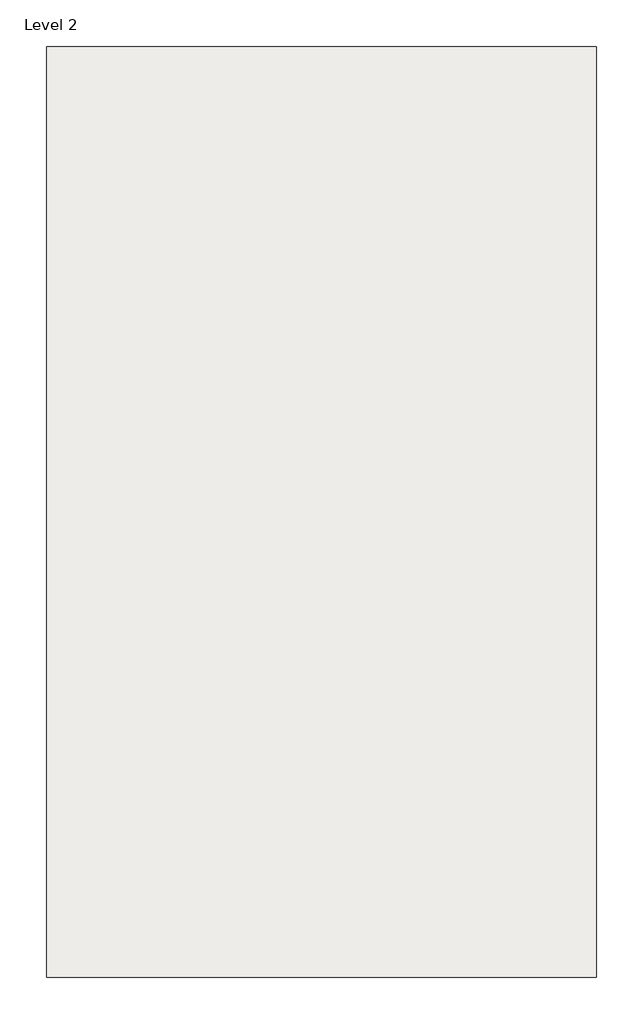
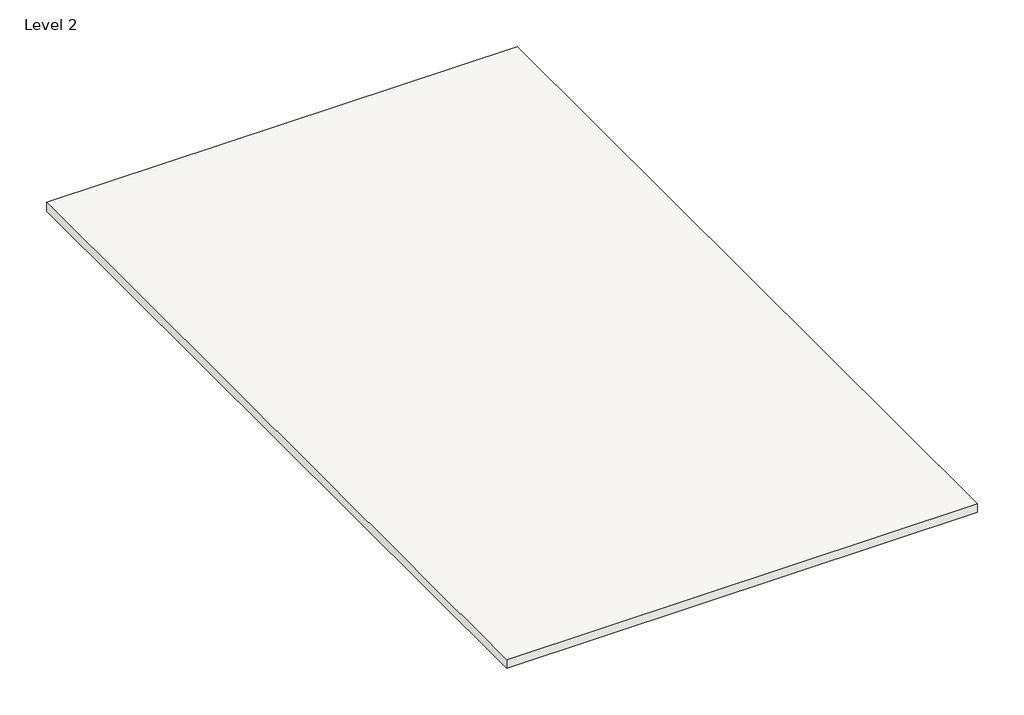
# One storey, incomplete: 1 roof.
"""IFC4 building model written with IfcOpenShell, lengths in millimetres."""

from ifc_helpers import new_model, si_unit, frame, origin, place, context, project, spatial, polyline, outline, extrude, element, save

model = new_model("IFC4")

# Units and contexts
model_context = context("Model", 3, world=origin())
ifc_project = project(units=[si_unit("LENGTHUNIT", "METRE", prefix="MILLI")], contexts=[model_context])

# Site, building, storey
site = spatial("IfcSite", under=ifc_project)
building = spatial("IfcBuilding", under=site)
storey = spatial("IfcBuildingStorey", under=building, Name="Level 2", Elevation=3048.0)

# Roof
placement = place(None, origin())
element("IfcRoof", 1, ObjectType="Generic - 12\"", at=placement, inside=storey, context=model_context, shape_type="SweptSolid", body=[
    extrude(outline(polyline([(-5222.940747, 7243.7935985), (2701.859253, 7243.7935985), (2701.859253, -6167.4064015), (-5222.940747, -6167.4064015), (-5222.940747, 7243.7935985)])), frame((0.0, 0.0, 3048.0), z_axis=(0.0, 0.0, 1.0), x_axis=(1.0, 0.0, 0.0)), (0.0, 0.0, 1.0), 152.4),
])

save(model, "model.ifc")

# Revit data of these elements
# Type "Generic - 12\""
#   Assembly Code = "B1020"
#   Layers, outside or top first: 0' - 6" no material (function 1)
# Element 1 (IfcRoof, "Generic - 12\"")
#   built-in parameter 1001705 = 10.5 (stored number, unit not read)
#   built-in parameter 1001710 = 33615
#   Phase Created = New Construction
#   Materials on its faces: "Default Roof", "Door - Panel"
# Materials
#   "Default Roof": colour RGB 88 101 114, transparency 0, Cost = 0
#   "Door - Panel": class "Wood", colour RGB 210 159 95, transparency 0, Cost = 0
